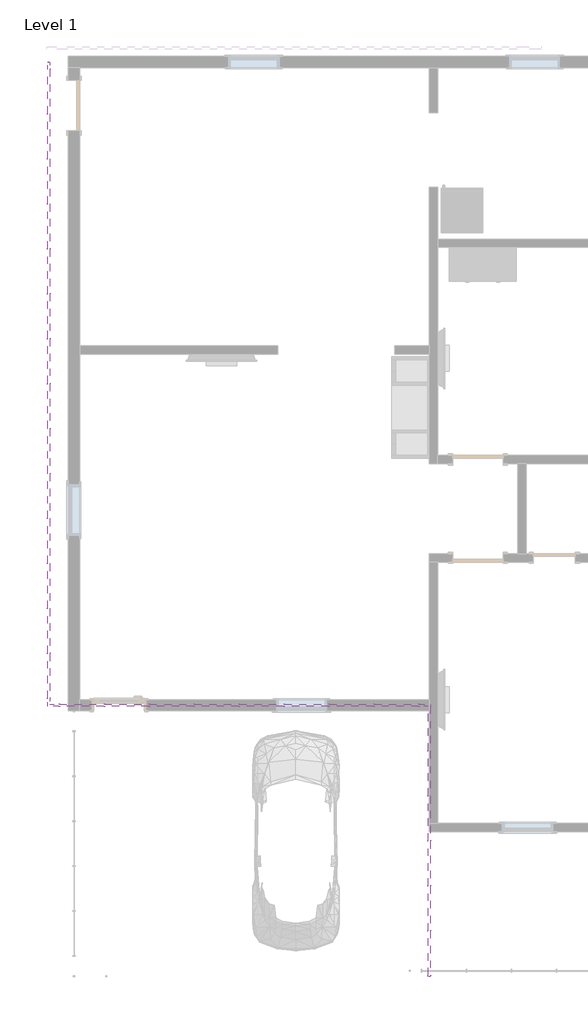
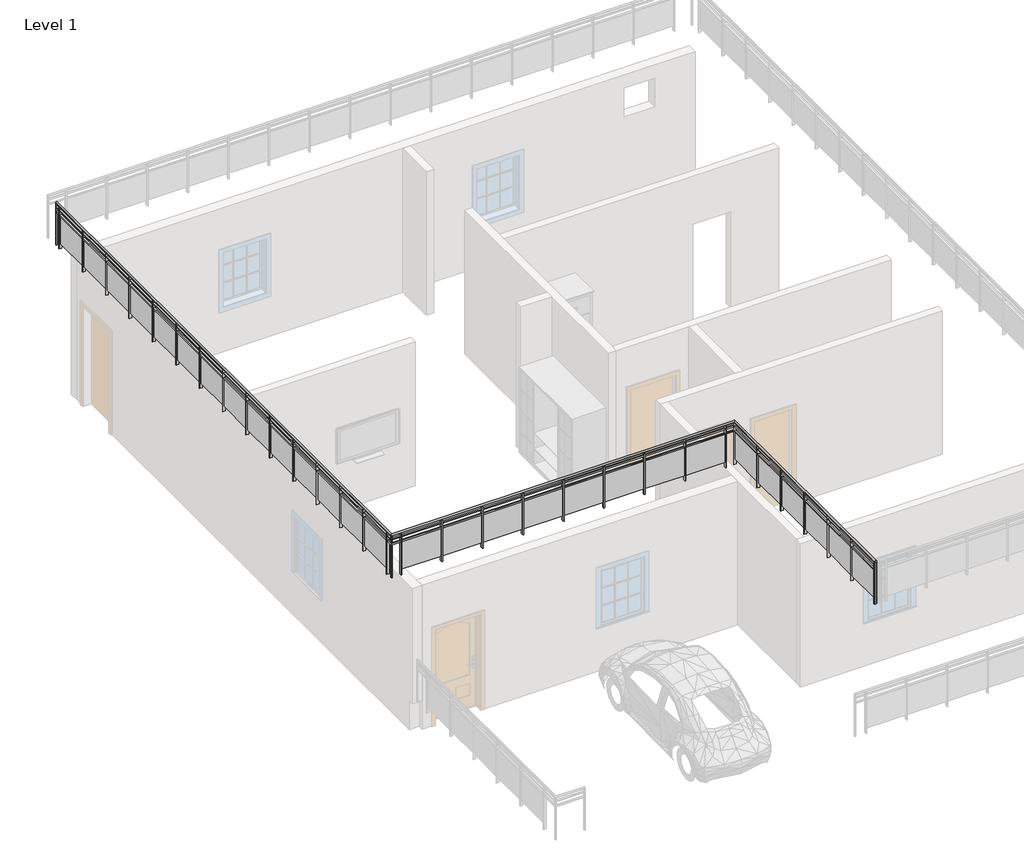
# One storey, part 3 of 5: 1 railing.
"""IFC4 building model written with IfcOpenShell, lengths in millimetres."""

from ifc_helpers import new_model, si_unit, frame, origin, place, context, project, spatial, polyline, circle_curve, ellipse_curve, outline, extrude, faceted_brep, element, save
from ifc_brep_helpers import plane_surface, cylinder_surface, advanced_brep

model = new_model("IFC4")

# Units and contexts
model_context = context("Model", 3, world=origin())
ifc_project = project(units=[si_unit("LENGTHUNIT", "METRE", prefix="MILLI")], contexts=[model_context])

# Site, building, storey
site = spatial("IfcSite", under=ifc_project)
building = spatial("IfcBuilding", under=site)
storey = spatial("IfcBuildingStorey", under=building, Name="Level 1", Elevation=0.0)

# Railing
placement = place(None, origin())
element("IfcRailing", 1, ObjectType="Glass Panel - Bottom Fill", at=placement, inside=storey, context=model_context, shape_type="SolidModel", body=[
    advanced_brep(
    [(-12693.4741134, 13899.2633056, 4248.15), (-12655.3741134, 13899.2633056, 4248.15), (-5810.0741134, -2636.1366944, 4248.15), (-5771.9741134, -2636.1366944, 4248.15), (-12693.4741134, 2247.0133056, 4248.15), (-12655.3741134, 2285.1133056, 4248.15), (-5810.0741134, 2247.0133056, 4248.15), (-5771.9741134, 2285.1133056, 4248.15)],
    [
        (0, 1, circle_curve(frame((-12674.4241134, 13899.2633056, 4248.15), z_axis=(0.0, 1.0, 0.0), x_axis=(1.0, 0.0, 0.0)), 19.05)),
        (1, 0, circle_curve(frame((-12674.4241134, 13899.2633056, 4248.15), z_axis=(0.0, 1.0, 0.0), x_axis=(1.0, 0.0, 0.0)), 19.05)),
        (2, 3, circle_curve(frame((-5791.0241134, -2636.1366944, 4248.15), z_axis=(0.0, -1.0, 0.0), x_axis=(1.0, 0.0, 0.0)), 19.05)),
        (3, 2, circle_curve(frame((-5791.0241134, -2636.1366944, 4248.15), z_axis=(0.0, -1.0, 0.0), x_axis=(1.0, 0.0, 0.0)), 19.05)),
        (0, 4),
        (4, 5, ellipse_curve(frame((-12674.4241134, 2266.0633056, 4248.15), z_axis=(-0.7071067811865458, 0.7071067811865492, 0.0), x_axis=(0.7071067811865491, 0.7071067811865458, 0.0)), 26.9407684, 19.05)),
        (5, 1),
        (5, 4, ellipse_curve(frame((-12674.4241134, 2266.0633056, 4248.15), z_axis=(-0.7071067811865458, 0.7071067811865492, 0.0), x_axis=(0.7071067811865491, 0.7071067811865458, 0.0)), 26.9407684, 19.05)),
        (4, 6),
        (6, 7, ellipse_curve(frame((-5791.0241134, 2266.0633056, 4248.15), z_axis=(-0.7071067811865458, 0.7071067811865492, 0.0), x_axis=(-0.7071067811865492, -0.7071067811865457, 0.0)), 26.9407684, 19.05)),
        (7, 5),
        (7, 6, ellipse_curve(frame((-5791.0241134, 2266.0633056, 4248.15), z_axis=(-0.7071067811865458, 0.7071067811865492, 0.0), x_axis=(-0.7071067811865492, -0.7071067811865457, 0.0)), 26.9407684, 19.05)),
        (6, 2),
        (3, 7),
    ],
    [
        plane_surface(frame((-12674.4241134, 13899.2633056, 4267.2), z_axis=(0.0, 1.0, 0.0), x_axis=(0.0, 0.0, -1.0))),
        plane_surface(frame((-5791.0241134, -2636.1366944, 4267.2), z_axis=(0.0, -1.0, 0.0), x_axis=(0.0, 0.0, -1.0))),
        cylinder_surface(frame((-12674.4241134, 13899.2633056, 4248.15), z_axis=(0.0, 1.0, 0.0), x_axis=(1.0, 0.0, 0.0)), 19.05),
        cylinder_surface(frame((-12674.4241134, 2266.0633056, 4248.15), z_axis=(-1.0, 0.0, 0.0), x_axis=(0.0, 1.0, 0.0)), 19.05),
        cylinder_surface(frame((-5791.0241134, 2266.0633056, 4248.15), z_axis=(0.0, 1.0, 0.0), x_axis=(1.0, 0.0, 0.0)), 19.05),
    ],
    [
        (0, [[1, 2]]),
        (1, [[3, 4]]),
        (2, [[-1, 5, 6, 7]]),
        (2, [[-2, -7, 8, -5]]),
        (3, [[-6, 9, 10, 11]]),
        (3, [[-8, -11, 12, -9]]),
        (4, [[-10, 13, -4, 14]]),
        (4, [[-12, -14, -3, -13]]),
    ],
),
    faceted_brep([(-12687.1241134, 13899.2633056, 4178.3), (-12661.7241134, 13899.2633056, 4178.3), (-12661.7241134, 13899.2633056, 4152.9), (-12687.1241134, 13899.2633056, 4152.9), (-12687.1241134, 2253.3633056, 4178.3), (-12661.7241134, 2278.7633056, 4178.3), (-12661.7241134, 2278.7633056, 4152.9), (-12687.1241134, 2253.3633056, 4152.9), (-5803.7241134, 2253.3633056, 4178.3), (-5778.3241134, 2278.7633056, 4178.3), (-5778.3241134, 2278.7633056, 4152.9), (-5803.7241134, 2253.3633056, 4152.9), (-5803.7241134, -2636.1366944, 4178.3), (-5803.7241134, -2636.1366944, 4152.9), (-5778.3241134, -2636.1366944, 4152.9), (-5778.3241134, -2636.1366944, 4178.3)], [[[0, 1, 2, 3]], [[1, 0, 4, 5]], [[2, 1, 5, 6]], [[3, 2, 6, 7]], [[0, 3, 7, 4]], [[5, 4, 8, 9]], [[6, 5, 9, 10]], [[7, 6, 10, 11]], [[4, 7, 11, 8]], [[12, 13, 14, 15]], [[9, 8, 12, 15]], [[10, 9, 15, 14]], [[11, 10, 14, 13]], [[8, 11, 13, 12]]]),
    faceted_brep([(-12687.1241134, 13899.2633056, 4076.7), (-12661.7241134, 13899.2633056, 4076.7), (-12661.7241134, 13899.2633056, 4051.3), (-12687.1241134, 13899.2633056, 4051.3), (-12687.1241134, 2253.3633056, 4076.7), (-12661.7241134, 2278.7633056, 4076.7), (-12661.7241134, 2278.7633056, 4051.3), (-12687.1241134, 2253.3633056, 4051.3), (-5803.7241134, 2253.3633056, 4076.7), (-5778.3241134, 2278.7633056, 4076.7), (-5778.3241134, 2278.7633056, 4051.3), (-5803.7241134, 2253.3633056, 4051.3), (-5803.7241134, -2636.1366944, 4076.7), (-5803.7241134, -2636.1366944, 4051.3), (-5778.3241134, -2636.1366944, 4051.3), (-5778.3241134, -2636.1366944, 4076.7)], [[[0, 1, 2, 3]], [[1, 0, 4, 5]], [[2, 1, 5, 6]], [[3, 2, 6, 7]], [[0, 3, 7, 4]], [[5, 4, 8, 9]], [[6, 5, 9, 10]], [[7, 6, 10, 11]], [[4, 7, 11, 8]], [[12, 13, 14, 15]], [[9, 8, 12, 15]], [[10, 9, 15, 14]], [[11, 10, 14, 13]], [[8, 11, 13, 12]]]),
    extrude(outline(polyline([(-5816.4241134, -2617.0866944), (-5765.6241134, -2617.0866944), (-5765.6241134, -2629.7866944), (-5816.4241134, -2629.7866944), (-5816.4241134, -2617.0866944)])), frame((0.0, 0.0, 3352.8), z_axis=(0.0, 0.0, 1.0), x_axis=(1.0, 0.0, 0.0)), (0.0, 0.0, 1.0), 876.3),
    extrude(outline(polyline([(-5784.4889564, -1810.6366944), (-5784.4889564, -2623.4366944), (-5790.8389564, -2623.4366944), (-5790.8389564, -1810.6366944), (-5784.4889564, -1810.6366944)])), frame((0.0, 0.0, 3454.4), z_axis=(0.0, 0.0, 1.0), x_axis=(1.0, 0.0, 0.0)), (0.0, 0.0, 1.0), 596.9),
    extrude(outline(polyline([(-5816.4241134, -1804.2866944), (-5765.6241134, -1804.2866944), (-5765.6241134, -1816.9866944), (-5816.4241134, -1816.9866944), (-5816.4241134, -1804.2866944)])), frame((0.0, 0.0, 3352.8), z_axis=(0.0, 0.0, 1.0), x_axis=(1.0, 0.0, 0.0)), (0.0, 0.0, 1.0), 876.3),
    extrude(outline(polyline([(-5784.4889564, -997.8366944), (-5784.4889564, -1810.6366944), (-5790.8389564, -1810.6366944), (-5790.8389564, -997.8366944), (-5784.4889564, -997.8366944)])), frame((0.0, 0.0, 3454.4), z_axis=(0.0, 0.0, 1.0), x_axis=(1.0, 0.0, 0.0)), (0.0, 0.0, 1.0), 596.9),
    extrude(outline(polyline([(-5816.4241134, -991.4866944), (-5765.6241134, -991.4866944), (-5765.6241134, -1004.1866944), (-5816.4241134, -1004.1866944), (-5816.4241134, -991.4866944)])), frame((0.0, 0.0, 3352.8), z_axis=(0.0, 0.0, 1.0), x_axis=(1.0, 0.0, 0.0)), (0.0, 0.0, 1.0), 876.3),
    extrude(outline(polyline([(-5784.4889564, -185.0366944), (-5784.4889564, -997.8366944), (-5790.8389564, -997.8366944), (-5790.8389564, -185.0366944), (-5784.4889564, -185.0366944)])), frame((0.0, 0.0, 3454.4), z_axis=(0.0, 0.0, 1.0), x_axis=(1.0, 0.0, 0.0)), (0.0, 0.0, 1.0), 596.9),
    extrude(outline(polyline([(-5816.4241134, -178.6866944), (-5765.6241134, -178.6866944), (-5765.6241134, -191.3866944), (-5816.4241134, -191.3866944), (-5816.4241134, -178.6866944)])), frame((0.0, 0.0, 3352.8), z_axis=(0.0, 0.0, 1.0), x_axis=(1.0, 0.0, 0.0)), (0.0, 0.0, 1.0), 876.3),
    extrude(outline(polyline([(-5784.4889564, 627.7633056), (-5784.4889564, -185.0366944), (-5790.8389564, -185.0366944), (-5790.8389564, 627.7633056), (-5784.4889564, 627.7633056)])), frame((0.0, 0.0, 3454.4), z_axis=(0.0, 0.0, 1.0), x_axis=(1.0, 0.0, 0.0)), (0.0, 0.0, 1.0), 596.9),
    extrude(outline(polyline([(-5816.4241134, 634.1133056), (-5765.6241134, 634.1133056), (-5765.6241134, 621.4133056), (-5816.4241134, 621.4133056), (-5816.4241134, 634.1133056)])), frame((0.0, 0.0, 3352.8), z_axis=(0.0, 0.0, 1.0), x_axis=(1.0, 0.0, 0.0)), (0.0, 0.0, 1.0), 876.3),
    extrude(outline(polyline([(-5784.4889564, 1440.5633056), (-5784.4889564, 627.7633056), (-5790.8389564, 627.7633056), (-5790.8389564, 1440.5633056), (-5784.4889564, 1440.5633056)])), frame((0.0, 0.0, 3454.4), z_axis=(0.0, 0.0, 1.0), x_axis=(1.0, 0.0, 0.0)), (0.0, 0.0, 1.0), 596.9),
    extrude(outline(polyline([(-5816.4241134, 1446.9133056), (-5765.6241134, 1446.9133056), (-5765.6241134, 1434.2133056), (-5816.4241134, 1434.2133056), (-5816.4241134, 1446.9133056)])), frame((0.0, 0.0, 3352.8), z_axis=(0.0, 0.0, 1.0), x_axis=(1.0, 0.0, 0.0)), (0.0, 0.0, 1.0), 876.3),
    extrude(outline(polyline([(-5784.4889564, 2253.3633056), (-5784.4889564, 1440.5633056), (-5790.8389564, 1440.5633056), (-5790.8389564, 2253.3633056), (-5784.4889564, 2253.3633056)])), frame((0.0, 0.0, 3454.4), z_axis=(0.0, 0.0, 1.0), x_axis=(1.0, 0.0, 0.0)), (0.0, 0.0, 1.0), 596.9),
    extrude(outline(polyline([(-5816.4241134, 2259.7133056), (-5765.6241134, 2259.7133056), (-5765.6241134, 2247.0133056), (-5816.4241134, 2247.0133056), (-5816.4241134, 2259.7133056)])), frame((0.0, 0.0, 3352.8), z_axis=(0.0, 0.0, 1.0), x_axis=(1.0, 0.0, 0.0)), (0.0, 0.0, 1.0), 876.3),
    extrude(outline(polyline([(-5987.8741134, 2240.6633056), (-5987.8741134, 2291.4633056), (-5975.1741134, 2291.4633056), (-5975.1741134, 2240.6633056), (-5987.8741134, 2240.6633056)])), frame((0.0, 0.0, 3352.8), z_axis=(0.0, 0.0, 1.0), x_axis=(1.0, 0.0, 0.0)), (0.0, 0.0, 1.0), 876.3),
    extrude(outline(polyline([(-6794.3241134, 2272.5984626), (-5981.5241134, 2272.5984626), (-5981.5241134, 2266.2484626), (-6794.3241134, 2266.2484626), (-6794.3241134, 2272.5984626)])), frame((0.0, 0.0, 3454.4), z_axis=(0.0, 0.0, 1.0), x_axis=(1.0, 0.0, 0.0)), (0.0, 0.0, 1.0), 596.9),
    extrude(outline(polyline([(-6800.6741134, 2240.6633056), (-6800.6741134, 2291.4633056), (-6787.9741134, 2291.4633056), (-6787.9741134, 2240.6633056), (-6800.6741134, 2240.6633056)])), frame((0.0, 0.0, 3352.8), z_axis=(0.0, 0.0, 1.0), x_axis=(1.0, 0.0, 0.0)), (0.0, 0.0, 1.0), 876.3),
    extrude(outline(polyline([(-7607.1241134, 2272.5984626), (-6794.3241134, 2272.5984626), (-6794.3241134, 2266.2484626), (-7607.1241134, 2266.2484626), (-7607.1241134, 2272.5984626)])), frame((0.0, 0.0, 3454.4), z_axis=(0.0, 0.0, 1.0), x_axis=(1.0, 0.0, 0.0)), (0.0, 0.0, 1.0), 596.9),
    extrude(outline(polyline([(-7613.4741134, 2240.6633056), (-7613.4741134, 2291.4633056), (-7600.7741134, 2291.4633056), (-7600.7741134, 2240.6633056), (-7613.4741134, 2240.6633056)])), frame((0.0, 0.0, 3352.8), z_axis=(0.0, 0.0, 1.0), x_axis=(1.0, 0.0, 0.0)), (0.0, 0.0, 1.0), 876.3),
    extrude(outline(polyline([(-8419.9241134, 2272.5984626), (-7607.1241134, 2272.5984626), (-7607.1241134, 2266.2484626), (-8419.9241134, 2266.2484626), (-8419.9241134, 2272.5984626)])), frame((0.0, 0.0, 3454.4), z_axis=(0.0, 0.0, 1.0), x_axis=(1.0, 0.0, 0.0)), (0.0, 0.0, 1.0), 596.9),
    extrude(outline(polyline([(-8426.2741134, 2240.6633056), (-8426.2741134, 2291.4633056), (-8413.5741134, 2291.4633056), (-8413.5741134, 2240.6633056), (-8426.2741134, 2240.6633056)])), frame((0.0, 0.0, 3352.8), z_axis=(0.0, 0.0, 1.0), x_axis=(1.0, 0.0, 0.0)), (0.0, 0.0, 1.0), 876.3),
    extrude(outline(polyline([(-9232.7241134, 2272.5984626), (-8419.9241134, 2272.5984626), (-8419.9241134, 2266.2484626), (-9232.7241134, 2266.2484626), (-9232.7241134, 2272.5984626)])), frame((0.0, 0.0, 3454.4), z_axis=(0.0, 0.0, 1.0), x_axis=(1.0, 0.0, 0.0)), (0.0, 0.0, 1.0), 596.9),
    extrude(outline(polyline([(-9239.0741134, 2240.6633056), (-9239.0741134, 2291.4633056), (-9226.3741134, 2291.4633056), (-9226.3741134, 2240.6633056), (-9239.0741134, 2240.6633056)])), frame((0.0, 0.0, 3352.8), z_axis=(0.0, 0.0, 1.0), x_axis=(1.0, 0.0, 0.0)), (0.0, 0.0, 1.0), 876.3),
    extrude(outline(polyline([(-10045.5241134, 2272.5984626), (-9232.7241134, 2272.5984626), (-9232.7241134, 2266.2484626), (-10045.5241134, 2266.2484626), (-10045.5241134, 2272.5984626)])), frame((0.0, 0.0, 3454.4), z_axis=(0.0, 0.0, 1.0), x_axis=(1.0, 0.0, 0.0)), (0.0, 0.0, 1.0), 596.9),
    extrude(outline(polyline([(-10051.8741134, 2240.6633056), (-10051.8741134, 2291.4633056), (-10039.1741134, 2291.4633056), (-10039.1741134, 2240.6633056), (-10051.8741134, 2240.6633056)])), frame((0.0, 0.0, 3352.8), z_axis=(0.0, 0.0, 1.0), x_axis=(1.0, 0.0, 0.0)), (0.0, 0.0, 1.0), 876.3),
    extrude(outline(polyline([(-10858.3241134, 2272.5984626), (-10045.5241134, 2272.5984626), (-10045.5241134, 2266.2484626), (-10858.3241134, 2266.2484626), (-10858.3241134, 2272.5984626)])), frame((0.0, 0.0, 3454.4), z_axis=(0.0, 0.0, 1.0), x_axis=(1.0, 0.0, 0.0)), (0.0, 0.0, 1.0), 596.9),
    extrude(outline(polyline([(-10864.6741134, 2240.6633056), (-10864.6741134, 2291.4633056), (-10851.9741134, 2291.4633056), (-10851.9741134, 2240.6633056), (-10864.6741134, 2240.6633056)])), frame((0.0, 0.0, 3352.8), z_axis=(0.0, 0.0, 1.0), x_axis=(1.0, 0.0, 0.0)), (0.0, 0.0, 1.0), 876.3),
    extrude(outline(polyline([(-11671.1241134, 2272.5984626), (-10858.3241134, 2272.5984626), (-10858.3241134, 2266.2484626), (-11671.1241134, 2266.2484626), (-11671.1241134, 2272.5984626)])), frame((0.0, 0.0, 3454.4), z_axis=(0.0, 0.0, 1.0), x_axis=(1.0, 0.0, 0.0)), (0.0, 0.0, 1.0), 596.9),
    extrude(outline(polyline([(-11677.4741134, 2240.6633056), (-11677.4741134, 2291.4633056), (-11664.7741134, 2291.4633056), (-11664.7741134, 2240.6633056), (-11677.4741134, 2240.6633056)])), frame((0.0, 0.0, 3352.8), z_axis=(0.0, 0.0, 1.0), x_axis=(1.0, 0.0, 0.0)), (0.0, 0.0, 1.0), 876.3),
    extrude(outline(polyline([(-12483.9241134, 2272.5984626), (-11671.1241134, 2272.5984626), (-11671.1241134, 2266.2484626), (-12483.9241134, 2266.2484626), (-12483.9241134, 2272.5984626)])), frame((0.0, 0.0, 3454.4), z_axis=(0.0, 0.0, 1.0), x_axis=(1.0, 0.0, 0.0)), (0.0, 0.0, 1.0), 596.9),
    extrude(outline(polyline([(-12490.2741134, 2240.6633056), (-12490.2741134, 2291.4633056), (-12477.5741134, 2291.4633056), (-12477.5741134, 2240.6633056), (-12490.2741134, 2240.6633056)])), frame((0.0, 0.0, 3352.8), z_axis=(0.0, 0.0, 1.0), x_axis=(1.0, 0.0, 0.0)), (0.0, 0.0, 1.0), 876.3),
    extrude(outline(polyline([(-12699.8241134, 2399.4133056), (-12649.0241134, 2399.4133056), (-12649.0241134, 2386.7133056), (-12699.8241134, 2386.7133056), (-12699.8241134, 2399.4133056)])), frame((0.0, 0.0, 3352.8), z_axis=(0.0, 0.0, 1.0), x_axis=(1.0, 0.0, 0.0)), (0.0, 0.0, 1.0), 876.3),
    extrude(outline(polyline([(-12667.8889564, 3205.8633056), (-12667.8889564, 2393.0633056), (-12674.2389564, 2393.0633056), (-12674.2389564, 3205.8633056), (-12667.8889564, 3205.8633056)])), frame((0.0, 0.0, 3454.4), z_axis=(0.0, 0.0, 1.0), x_axis=(1.0, 0.0, 0.0)), (0.0, 0.0, 1.0), 596.9),
    extrude(outline(polyline([(-12699.8241134, 3212.2133056), (-12649.0241134, 3212.2133056), (-12649.0241134, 3199.5133056), (-12699.8241134, 3199.5133056), (-12699.8241134, 3212.2133056)])), frame((0.0, 0.0, 3352.8), z_axis=(0.0, 0.0, 1.0), x_axis=(1.0, 0.0, 0.0)), (0.0, 0.0, 1.0), 876.3),
    extrude(outline(polyline([(-12667.8889564, 4018.6633056), (-12667.8889564, 3205.8633056), (-12674.2389564, 3205.8633056), (-12674.2389564, 4018.6633056), (-12667.8889564, 4018.6633056)])), frame((0.0, 0.0, 3454.4), z_axis=(0.0, 0.0, 1.0), x_axis=(1.0, 0.0, 0.0)), (0.0, 0.0, 1.0), 596.9),
    extrude(outline(polyline([(-12699.8241134, 4025.0133056), (-12649.0241134, 4025.0133056), (-12649.0241134, 4012.3133056), (-12699.8241134, 4012.3133056), (-12699.8241134, 4025.0133056)])), frame((0.0, 0.0, 3352.8), z_axis=(0.0, 0.0, 1.0), x_axis=(1.0, 0.0, 0.0)), (0.0, 0.0, 1.0), 876.3),
    extrude(outline(polyline([(-12667.8889564, 4831.4633056), (-12667.8889564, 4018.6633056), (-12674.2389564, 4018.6633056), (-12674.2389564, 4831.4633056), (-12667.8889564, 4831.4633056)])), frame((0.0, 0.0, 3454.4), z_axis=(0.0, 0.0, 1.0), x_axis=(1.0, 0.0, 0.0)), (0.0, 0.0, 1.0), 596.9),
    extrude(outline(polyline([(-12699.8241134, 4837.8133056), (-12649.0241134, 4837.8133056), (-12649.0241134, 4825.1133056), (-12699.8241134, 4825.1133056), (-12699.8241134, 4837.8133056)])), frame((0.0, 0.0, 3352.8), z_axis=(0.0, 0.0, 1.0), x_axis=(1.0, 0.0, 0.0)), (0.0, 0.0, 1.0), 876.3),
    extrude(outline(polyline([(-12667.8889564, 5644.2633056), (-12667.8889564, 4831.4633056), (-12674.2389564, 4831.4633056), (-12674.2389564, 5644.2633056), (-12667.8889564, 5644.2633056)])), frame((0.0, 0.0, 3454.4), z_axis=(0.0, 0.0, 1.0), x_axis=(1.0, 0.0, 0.0)), (0.0, 0.0, 1.0), 596.9),
    extrude(outline(polyline([(-12699.8241134, 5650.6133056), (-12649.0241134, 5650.6133056), (-12649.0241134, 5637.9133056), (-12699.8241134, 5637.9133056), (-12699.8241134, 5650.6133056)])), frame((0.0, 0.0, 3352.8), z_axis=(0.0, 0.0, 1.0), x_axis=(1.0, 0.0, 0.0)), (0.0, 0.0, 1.0), 876.3),
    extrude(outline(polyline([(-12667.8889564, 6457.0633056), (-12667.8889564, 5644.2633056), (-12674.2389564, 5644.2633056), (-12674.2389564, 6457.0633056), (-12667.8889564, 6457.0633056)])), frame((0.0, 0.0, 3454.4), z_axis=(0.0, 0.0, 1.0), x_axis=(1.0, 0.0, 0.0)), (0.0, 0.0, 1.0), 596.9),
    extrude(outline(polyline([(-12699.8241134, 6463.4133056), (-12649.0241134, 6463.4133056), (-12649.0241134, 6450.7133056), (-12699.8241134, 6450.7133056), (-12699.8241134, 6463.4133056)])), frame((0.0, 0.0, 3352.8), z_axis=(0.0, 0.0, 1.0), x_axis=(1.0, 0.0, 0.0)), (0.0, 0.0, 1.0), 876.3),
    extrude(outline(polyline([(-12667.8889564, 7269.8633056), (-12667.8889564, 6457.0633056), (-12674.2389564, 6457.0633056), (-12674.2389564, 7269.8633056), (-12667.8889564, 7269.8633056)])), frame((0.0, 0.0, 3454.4), z_axis=(0.0, 0.0, 1.0), x_axis=(1.0, 0.0, 0.0)), (0.0, 0.0, 1.0), 596.9),
    extrude(outline(polyline([(-12699.8241134, 7276.2133056), (-12649.0241134, 7276.2133056), (-12649.0241134, 7263.5133056), (-12699.8241134, 7263.5133056), (-12699.8241134, 7276.2133056)])), frame((0.0, 0.0, 3352.8), z_axis=(0.0, 0.0, 1.0), x_axis=(1.0, 0.0, 0.0)), (0.0, 0.0, 1.0), 876.3),
    extrude(outline(polyline([(-12667.8889564, 8082.6633056), (-12667.8889564, 7269.8633056), (-12674.2389564, 7269.8633056), (-12674.2389564, 8082.6633056), (-12667.8889564, 8082.6633056)])), frame((0.0, 0.0, 3454.4), z_axis=(0.0, 0.0, 1.0), x_axis=(1.0, 0.0, 0.0)), (0.0, 0.0, 1.0), 596.9),
    extrude(outline(polyline([(-12699.8241134, 8089.0133056), (-12649.0241134, 8089.0133056), (-12649.0241134, 8076.3133056), (-12699.8241134, 8076.3133056), (-12699.8241134, 8089.0133056)])), frame((0.0, 0.0, 3352.8), z_axis=(0.0, 0.0, 1.0), x_axis=(1.0, 0.0, 0.0)), (0.0, 0.0, 1.0), 876.3),
    extrude(outline(polyline([(-12667.8889564, 8895.4633056), (-12667.8889564, 8082.6633056), (-12674.2389564, 8082.6633056), (-12674.2389564, 8895.4633056), (-12667.8889564, 8895.4633056)])), frame((0.0, 0.0, 3454.4), z_axis=(0.0, 0.0, 1.0), x_axis=(1.0, 0.0, 0.0)), (0.0, 0.0, 1.0), 596.9),
    extrude(outline(polyline([(-12699.8241134, 8901.8133056), (-12649.0241134, 8901.8133056), (-12649.0241134, 8889.1133056), (-12699.8241134, 8889.1133056), (-12699.8241134, 8901.8133056)])), frame((0.0, 0.0, 3352.8), z_axis=(0.0, 0.0, 1.0), x_axis=(1.0, 0.0, 0.0)), (0.0, 0.0, 1.0), 876.3),
    extrude(outline(polyline([(-12667.8889564, 9708.2633056), (-12667.8889564, 8895.4633056), (-12674.2389564, 8895.4633056), (-12674.2389564, 9708.2633056), (-12667.8889564, 9708.2633056)])), frame((0.0, 0.0, 3454.4), z_axis=(0.0, 0.0, 1.0), x_axis=(1.0, 0.0, 0.0)), (0.0, 0.0, 1.0), 596.9),
    extrude(outline(polyline([(-12699.8241134, 9714.6133056), (-12649.0241134, 9714.6133056), (-12649.0241134, 9701.9133056), (-12699.8241134, 9701.9133056), (-12699.8241134, 9714.6133056)])), frame((0.0, 0.0, 3352.8), z_axis=(0.0, 0.0, 1.0), x_axis=(1.0, 0.0, 0.0)), (0.0, 0.0, 1.0), 876.3),
    extrude(outline(polyline([(-12667.8889564, 10521.0633056), (-12667.8889564, 9708.2633056), (-12674.2389564, 9708.2633056), (-12674.2389564, 10521.0633056), (-12667.8889564, 10521.0633056)])), frame((0.0, 0.0, 3454.4), z_axis=(0.0, 0.0, 1.0), x_axis=(1.0, 0.0, 0.0)), (0.0, 0.0, 1.0), 596.9),
    extrude(outline(polyline([(-12699.8241134, 10527.4133056), (-12649.0241134, 10527.4133056), (-12649.0241134, 10514.7133056), (-12699.8241134, 10514.7133056), (-12699.8241134, 10527.4133056)])), frame((0.0, 0.0, 3352.8), z_axis=(0.0, 0.0, 1.0), x_axis=(1.0, 0.0, 0.0)), (0.0, 0.0, 1.0), 876.3),
    extrude(outline(polyline([(-12667.8889564, 11333.8633056), (-12667.8889564, 10521.0633056), (-12674.2389564, 10521.0633056), (-12674.2389564, 11333.8633056), (-12667.8889564, 11333.8633056)])), frame((0.0, 0.0, 3454.4), z_axis=(0.0, 0.0, 1.0), x_axis=(1.0, 0.0, 0.0)), (0.0, 0.0, 1.0), 596.9),
    extrude(outline(polyline([(-12699.8241134, 11340.2133056), (-12649.0241134, 11340.2133056), (-12649.0241134, 11327.5133056), (-12699.8241134, 11327.5133056), (-12699.8241134, 11340.2133056)])), frame((0.0, 0.0, 3352.8), z_axis=(0.0, 0.0, 1.0), x_axis=(1.0, 0.0, 0.0)), (0.0, 0.0, 1.0), 876.3),
    extrude(outline(polyline([(-12667.8889564, 12146.6633056), (-12667.8889564, 11333.8633056), (-12674.2389564, 11333.8633056), (-12674.2389564, 12146.6633056), (-12667.8889564, 12146.6633056)])), frame((0.0, 0.0, 3454.4), z_axis=(0.0, 0.0, 1.0), x_axis=(1.0, 0.0, 0.0)), (0.0, 0.0, 1.0), 596.9),
    extrude(outline(polyline([(-12699.8241134, 12153.0133056), (-12649.0241134, 12153.0133056), (-12649.0241134, 12140.3133056), (-12699.8241134, 12140.3133056), (-12699.8241134, 12153.0133056)])), frame((0.0, 0.0, 3352.8), z_axis=(0.0, 0.0, 1.0), x_axis=(1.0, 0.0, 0.0)), (0.0, 0.0, 1.0), 876.3),
    extrude(outline(polyline([(-12667.8889564, 12959.4633056), (-12667.8889564, 12146.6633056), (-12674.2389564, 12146.6633056), (-12674.2389564, 12959.4633056), (-12667.8889564, 12959.4633056)])), frame((0.0, 0.0, 3454.4), z_axis=(0.0, 0.0, 1.0), x_axis=(1.0, 0.0, 0.0)), (0.0, 0.0, 1.0), 596.9),
    extrude(outline(polyline([(-12699.8241134, 12965.8133056), (-12649.0241134, 12965.8133056), (-12649.0241134, 12953.1133056), (-12699.8241134, 12953.1133056), (-12699.8241134, 12965.8133056)])), frame((0.0, 0.0, 3352.8), z_axis=(0.0, 0.0, 1.0), x_axis=(1.0, 0.0, 0.0)), (0.0, 0.0, 1.0), 876.3),
    extrude(outline(polyline([(-12667.8889564, 13772.2633056), (-12667.8889564, 12959.4633056), (-12674.2389564, 12959.4633056), (-12674.2389564, 13772.2633056), (-12667.8889564, 13772.2633056)])), frame((0.0, 0.0, 3454.4), z_axis=(0.0, 0.0, 1.0), x_axis=(1.0, 0.0, 0.0)), (0.0, 0.0, 1.0), 596.9),
    extrude(outline(polyline([(-12699.8241134, 13778.6133056), (-12649.0241134, 13778.6133056), (-12649.0241134, 13765.9133056), (-12699.8241134, 13765.9133056), (-12699.8241134, 13778.6133056)])), frame((0.0, 0.0, 3352.8), z_axis=(0.0, 0.0, 1.0), x_axis=(1.0, 0.0, 0.0)), (0.0, 0.0, 1.0), 876.3),
    extrude(outline(polyline([(-5800.5491134, 2256.5383056), (-5800.5491134, 2275.5883056), (-5781.4991134, 2275.5883056), (-5781.4991134, 2256.5383056), (-5800.5491134, 2256.5383056)])), frame((0.0, 0.0, 3352.8), z_axis=(0.0, 0.0, 1.0), x_axis=(1.0, 0.0, 0.0)), (0.0, 0.0, 1.0), 876.3),
    extrude(outline(polyline([(-12683.9491134, 2275.5883056), (-12664.8991134, 2275.5883056), (-12664.8991134, 2256.5383056), (-12683.9491134, 2256.5383056), (-12683.9491134, 2275.5883056)])), frame((0.0, 0.0, 3352.8), z_axis=(0.0, 0.0, 1.0), x_axis=(1.0, 0.0, 0.0)), (0.0, 0.0, 1.0), 876.3),
    extrude(outline(polyline([(-5800.5491134, -2623.4366944), (-5781.4991134, -2623.4366944), (-5781.4991134, -2642.4866944), (-5800.5491134, -2642.4866944), (-5800.5491134, -2623.4366944)])), frame((0.0, 0.0, 3352.8), z_axis=(0.0, 0.0, 1.0), x_axis=(1.0, 0.0, 0.0)), (0.0, 0.0, 1.0), 876.3),
    extrude(outline(polyline([(-12683.9491134, 13905.6133056), (-12664.8991134, 13905.6133056), (-12664.8991134, 13886.5633056), (-12683.9491134, 13886.5633056), (-12683.9491134, 13905.6133056)])), frame((0.0, 0.0, 3352.8), z_axis=(0.0, 0.0, 1.0), x_axis=(1.0, 0.0, 0.0)), (0.0, 0.0, 1.0), 876.3),
])

save(model, "model.ifc")

# Revit data of these elements
# Type "Glass Panel - Bottom Fill"
#   Assembly Code = "C2010400"
#   built-in parameter 1008612 = 0.0416667 (stored number, unit not read)
#   built-in parameter 1008611 = 0.0416667 (stored number, unit not read)
#   built-in parameter 1008609 = 0.333333 (stored number, unit not read)
#   built-in parameter 1008604 = 0.166667 (stored number, unit not read)
#   built-in parameter 1008603 = 0.166667 (stored number, unit not read)
#   Railing Height = 3' - 0"
#   built-in parameter 1008630 = 2
#   built-in parameter 1008610 = 2
#   built-in parameter 1008618 = Baluster - Square : 3/4"
# Element 1 (IfcRailing, "Glass Panel - Bottom Fill")
#   built-in parameter 1008621 = 11 (stored number, unit not read)
#   Phase Created = New Construction
#   Materials on its faces: "Glass"
# Materials
#   "Glass": class "Glass", colour RGB 0 128 192, transparency 0.75, Description = "Soda Lime Glass", Cost = 0
